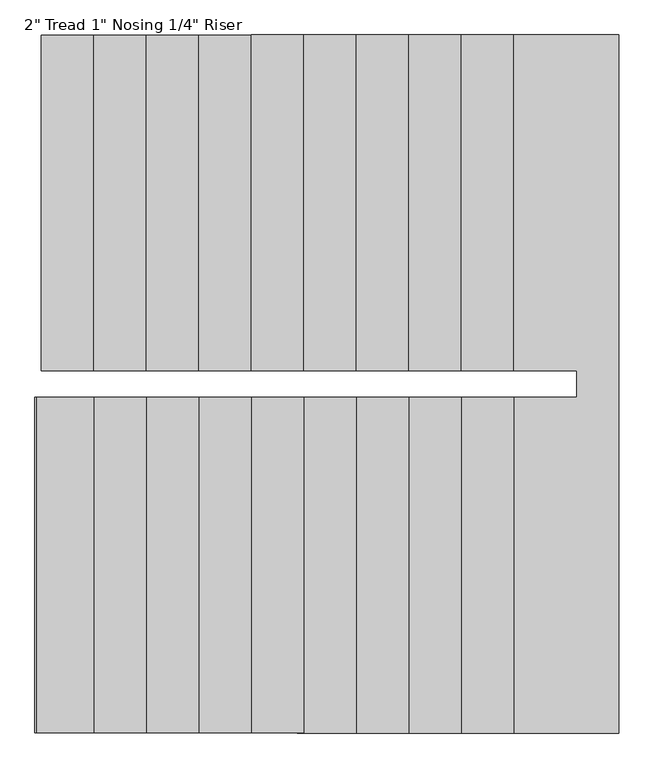
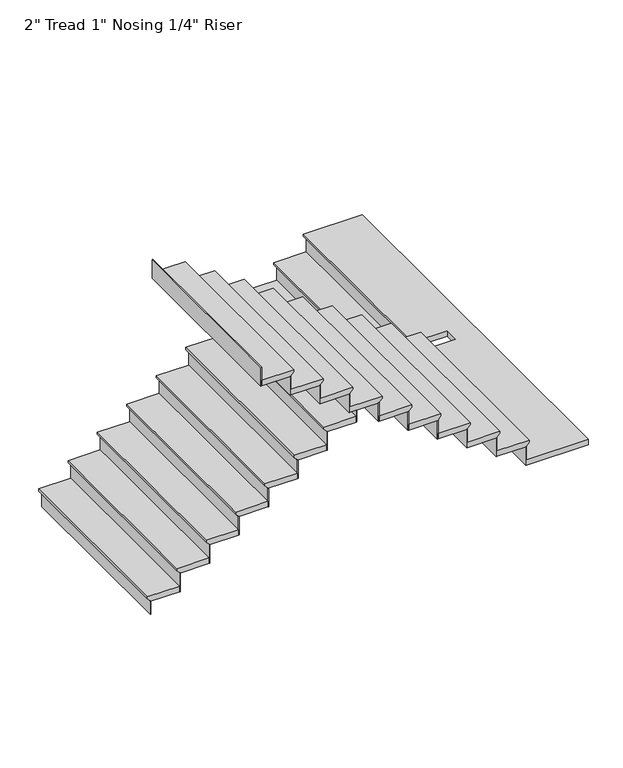
"""IFC4 building model written with IfcOpenShell, lengths in millimetres: stair flight geometry."""

from ifc_helpers import new_model, si_unit, origin, place, context, project, spatial, faceted_brep, source, transform, mapped, element, save


def stair_flight_0ebd5bc4(model_context):
    return source(origin(), model_context, "Body", "Brep", [
        faceted_brep([(-6414.1711241, 10106.9344295, 150.2833333), (-6414.1711241, 10106.9344295, 169.3333333), (-6414.1711241, 11732.5344295, 169.3333333), (-6414.1711241, 11732.5344295, 150.2833333), (-6388.7711241, 10106.9344295, 124.8833333), (-6388.7711241, 11732.5344295, 124.8833333), (-6134.7711241, 10106.9344295, 169.3333333), (-6134.7711241, 11732.5344295, 169.3333333), (-6388.7711241, 11732.5344295, 118.5333333), (-6134.7711241, 11732.5344295, 118.5333333), (-6134.7711241, 10106.9344295, 118.5333333), (-6388.7711241, 10106.9344295, 118.5333333)], [[[0, 1, 2, 3]], [[4, 0, 3, 5]], [[2, 1, 6, 7]], [[8, 9, 10, 11]], [[2, 7, 9, 8, 5, 3]], [[8, 11, 4, 5]], [[6, 1, 0, 4, 11, 10]], [[7, 6, 10, 9]]]),
        faceted_brep([(-6388.7711241, 10106.9344295, 118.5333333), (-6388.7711241, 10106.9344295, 0.0), (-6382.4211241, 10106.9344295, 0.0), (-6382.4211241, 10106.9344295, 118.5333333), (-6388.7711241, 11732.5344295, 118.5333333), (-6382.4211241, 11732.5344295, 118.5333333), (-6382.4211241, 11732.5344295, 0.0), (-6388.7711241, 11732.5344295, 0.0)], [[[0, 1, 2, 3]], [[4, 5, 6, 7]], [[1, 0, 4, 7]], [[2, 1, 7, 6]], [[3, 2, 6, 5]], [[0, 3, 5, 4]]]),
        faceted_brep([(-6134.7711241, 10106.9344295, 287.8666667), (-6134.7711241, 10106.9344295, 118.5333333), (-6128.4211241, 10106.9344295, 118.5333333), (-6128.4211241, 10106.9344295, 287.8666667), (-6134.7711241, 11732.5344295, 287.8666667), (-6128.4211241, 11732.5344295, 287.8666667), (-6128.4211241, 11732.5344295, 118.5333333), (-6134.7711241, 11732.5344295, 118.5333333)], [[[0, 1, 2, 3]], [[4, 5, 6, 7]], [[1, 0, 4, 7]], [[2, 1, 7, 6]], [[3, 2, 6, 5]], [[0, 3, 5, 4]]]),
        faceted_brep([(-6160.1711241, 11732.5344295, 338.6666667), (-6160.1711241, 10106.9344295, 338.6666667), (-5880.7711241, 10106.9344295, 338.6666667), (-5880.7711241, 11732.5344295, 338.6666667), (-6134.7711241, 11732.5344295, 287.8666667), (-5880.7711241, 11732.5344295, 287.8666667), (-5880.7711241, 10106.9344295, 287.8666667), (-6134.7711241, 10106.9344295, 287.8666667), (-6134.7711241, 11732.5344295, 294.2166667), (-6160.1711241, 11732.5344295, 319.6166667), (-6134.7711241, 10106.9344295, 294.2166667), (-6160.1711241, 10106.9344295, 319.6166667)], [[[0, 1, 2, 3]], [[4, 5, 6, 7]], [[0, 3, 5, 4, 8, 9]], [[4, 7, 10, 8]], [[2, 1, 11, 10, 7, 6]], [[3, 2, 6, 5]], [[11, 1, 0, 9]], [[10, 11, 9, 8]]]),
        faceted_brep([(-5880.7711241, 10106.9344295, 457.2), (-5880.7711241, 10106.9344295, 287.8666667), (-5874.4211241, 10106.9344295, 287.8666667), (-5874.4211241, 10106.9344295, 457.2), (-5880.7711241, 11732.5344295, 457.2), (-5874.4211241, 11732.5344295, 457.2), (-5874.4211241, 11732.5344295, 287.8666667), (-5880.7711241, 11732.5344295, 287.8666667)], [[[0, 1, 2, 3]], [[4, 5, 6, 7]], [[1, 0, 4, 7]], [[2, 1, 7, 6]], [[3, 2, 6, 5]], [[0, 3, 5, 4]]]),
        faceted_brep([(-5906.1711241, 11732.5344295, 508.0), (-5906.1711241, 10106.9344295, 508.0), (-5626.7711241, 10106.9344295, 508.0), (-5626.7711241, 11732.5344295, 508.0), (-5880.7711241, 11732.5344295, 457.2), (-5626.7711241, 11732.5344295, 457.2), (-5626.7711241, 10106.9344295, 457.2), (-5880.7711241, 10106.9344295, 457.2), (-5880.7711241, 11732.5344295, 463.55), (-5906.1711241, 11732.5344295, 488.95), (-5880.7711241, 10106.9344295, 463.55), (-5906.1711241, 10106.9344295, 488.95)], [[[0, 1, 2, 3]], [[4, 5, 6, 7]], [[0, 3, 5, 4, 8, 9]], [[4, 7, 10, 8]], [[2, 1, 11, 10, 7, 6]], [[3, 2, 6, 5]], [[11, 1, 0, 9]], [[10, 11, 9, 8]]]),
        faceted_brep([(-5626.7711241, 10106.9344295, 626.5333333), (-5626.7711241, 10106.9344295, 457.2), (-5620.4211241, 10106.9344295, 457.2), (-5620.4211241, 10106.9344295, 626.5333333), (-5626.7711241, 11732.5344295, 626.5333333), (-5620.4211241, 11732.5344295, 626.5333333), (-5620.4211241, 11732.5344295, 457.2), (-5626.7711241, 11732.5344295, 457.2)], [[[0, 1, 2, 3]], [[4, 5, 6, 7]], [[1, 0, 4, 7]], [[2, 1, 7, 6]], [[3, 2, 6, 5]], [[0, 3, 5, 4]]]),
        faceted_brep([(-5652.1711241, 11732.5344295, 677.3333333), (-5652.1711241, 10106.9344295, 677.3333333), (-5372.7711241, 10106.9344295, 677.3333333), (-5372.7711241, 11732.5344295, 677.3333333), (-5626.7711241, 11732.5344295, 626.5333333), (-5372.7711241, 11732.5344295, 626.5333333), (-5372.7711241, 10106.9344295, 626.5333333), (-5626.7711241, 10106.9344295, 626.5333333), (-5626.7711241, 11732.5344295, 632.8833333), (-5652.1711241, 11732.5344295, 658.2833333), (-5626.7711241, 10106.9344295, 632.8833333), (-5652.1711241, 10106.9344295, 658.2833333)], [[[0, 1, 2, 3]], [[4, 5, 6, 7]], [[0, 3, 5, 4, 8, 9]], [[4, 7, 10, 8]], [[2, 1, 11, 10, 7, 6]], [[3, 2, 6, 5]], [[11, 1, 0, 9]], [[10, 11, 9, 8]]]),
        faceted_brep([(-5372.7711241, 10106.9344295, 795.8666667), (-5372.7711241, 10106.9344295, 626.5333333), (-5366.4211241, 10106.9344295, 626.5333333), (-5366.4211241, 10106.9344295, 795.8666667), (-5372.7711241, 11732.5344295, 795.8666667), (-5366.4211241, 11732.5344295, 795.8666667), (-5366.4211241, 11732.5344295, 626.5333333), (-5372.7711241, 11732.5344295, 626.5333333)], [[[0, 1, 2, 3]], [[4, 5, 6, 7]], [[1, 0, 4, 7]], [[2, 1, 7, 6]], [[3, 2, 6, 5]], [[0, 3, 5, 4]]]),
        faceted_brep([(-5398.1711241, 11732.5344295, 846.6666667), (-5398.1711241, 10106.9344295, 846.6666667), (-5118.7711241, 10106.9344295, 846.6666667), (-5118.7711241, 11732.5344295, 846.6666667), (-5372.7711241, 11732.5344295, 795.8666667), (-5118.7711241, 11732.5344295, 795.8666667), (-5118.7711241, 10106.9344295, 795.8666667), (-5372.7711241, 10106.9344295, 795.8666667), (-5372.7711241, 11732.5344295, 802.2166667), (-5398.1711241, 11732.5344295, 827.6166667), (-5372.7711241, 10106.9344295, 802.2166667), (-5398.1711241, 10106.9344295, 827.6166667)], [[[0, 1, 2, 3]], [[4, 5, 6, 7]], [[0, 3, 5, 4, 8, 9]], [[4, 7, 10, 8]], [[2, 1, 11, 10, 7, 6]], [[3, 2, 6, 5]], [[11, 1, 0, 9]], [[10, 11, 9, 8]]]),
        faceted_brep([(-5118.7711241, 10106.9344295, 965.2), (-5118.7711241, 10106.9344295, 795.8666667), (-5112.4211241, 10106.9344295, 795.8666667), (-5112.4211241, 10106.9344295, 965.2), (-5118.7711241, 11732.5344295, 965.2), (-5112.4211241, 11732.5344295, 965.2), (-5112.4211241, 11732.5344295, 795.8666667), (-5118.7711241, 11732.5344295, 795.8666667)], [[[0, 1, 2, 3]], [[4, 5, 6, 7]], [[1, 0, 4, 7]], [[2, 1, 7, 6]], [[3, 2, 6, 5]], [[0, 3, 5, 4]]]),
        faceted_brep([(-5144.1711241, 11732.5344295, 1016.0), (-5144.1711241, 10106.9344295, 1016.0), (-4864.7711241, 10106.9344295, 1016.0), (-4864.7711241, 11732.5344295, 1016.0), (-5118.7711241, 11732.5344295, 965.2), (-4864.7711241, 11732.5344295, 965.2), (-4864.7711241, 10106.9344295, 965.2), (-5118.7711241, 10106.9344295, 965.2), (-5118.7711241, 11732.5344295, 971.55), (-5144.1711241, 11732.5344295, 996.95), (-5118.7711241, 10106.9344295, 971.55), (-5144.1711241, 10106.9344295, 996.95)], [[[0, 1, 2, 3]], [[4, 5, 6, 7]], [[0, 3, 5, 4, 8, 9]], [[4, 7, 10, 8]], [[2, 1, 11, 10, 7, 6]], [[3, 2, 6, 5]], [[11, 1, 0, 9]], [[10, 11, 9, 8]]]),
        faceted_brep([(-4864.7711241, 10106.9344295, 1134.5333333), (-4864.7711241, 10106.9344295, 965.2), (-4858.4211241, 10106.9344295, 965.2), (-4858.4211241, 10106.9344295, 1134.5333333), (-4864.7711241, 11732.5344295, 1134.5333333), (-4858.4211241, 11732.5344295, 1134.5333333), (-4858.4211241, 11732.5344295, 965.2), (-4864.7711241, 11732.5344295, 965.2)], [[[0, 1, 2, 3]], [[4, 5, 6, 7]], [[1, 0, 4, 7]], [[2, 1, 7, 6]], [[3, 2, 6, 5]], [[0, 3, 5, 4]]]),
        faceted_brep([(-4890.1711241, 11732.5344295, 1185.3333333), (-4890.1711241, 10106.9344295, 1185.3333333), (-4610.7711241, 10106.9344295, 1185.3333333), (-4610.7711241, 11732.5344295, 1185.3333333), (-4864.7711241, 11732.5344295, 1134.5333333), (-4610.7711241, 11732.5344295, 1134.5333333), (-4610.7711241, 10106.9344295, 1134.5333333), (-4864.7711241, 10106.9344295, 1134.5333333), (-4864.7711241, 11732.5344295, 1140.8833333), (-4890.1711241, 11732.5344295, 1166.2833333), (-4864.7711241, 10106.9344295, 1140.8833333), (-4890.1711241, 10106.9344295, 1166.2833333)], [[[0, 1, 2, 3]], [[4, 5, 6, 7]], [[0, 3, 5, 4, 8, 9]], [[4, 7, 10, 8]], [[2, 1, 11, 10, 7, 6]], [[3, 2, 6, 5]], [[11, 1, 0, 9]], [[10, 11, 9, 8]]]),
        faceted_brep([(-4610.7711241, 10106.9344295, 1303.8666667), (-4610.7711241, 10106.9344295, 1134.5333333), (-4604.4211241, 10106.9344295, 1134.5333333), (-4604.4211241, 10106.9344295, 1303.8666667), (-4610.7711241, 11732.5344295, 1303.8666667), (-4604.4211241, 11732.5344295, 1303.8666667), (-4604.4211241, 11732.5344295, 1134.5333333), (-4610.7711241, 11732.5344295, 1134.5333333)], [[[0, 1, 2, 3]], [[4, 5, 6, 7]], [[1, 0, 4, 7]], [[2, 1, 7, 6]], [[3, 2, 6, 5]], [[0, 3, 5, 4]]]),
        faceted_brep([(-4636.1711241, 11732.5344295, 1354.6666667), (-4636.1711241, 10106.9344295, 1354.6666667), (-4356.7711241, 10106.9344295, 1354.6666667), (-4356.7711241, 11732.5344295, 1354.6666667), (-4610.7711241, 11732.5344295, 1303.8666667), (-4356.7711241, 11732.5344295, 1303.8666667), (-4356.7711241, 10106.9344295, 1303.8666667), (-4610.7711241, 10106.9344295, 1303.8666667), (-4610.7711241, 11732.5344295, 1310.2166667), (-4636.1711241, 11732.5344295, 1335.6166667), (-4610.7711241, 10106.9344295, 1310.2166667), (-4636.1711241, 10106.9344295, 1335.6166667)], [[[0, 1, 2, 3]], [[4, 5, 6, 7]], [[0, 3, 5, 4, 8, 9]], [[4, 7, 10, 8]], [[2, 1, 11, 10, 7, 6]], [[3, 2, 6, 5]], [[11, 1, 0, 9]], [[10, 11, 9, 8]]]),
        faceted_brep([(-4356.7711241, 10106.9344295, 1473.2), (-4356.7711241, 10106.9344295, 1303.8666667), (-4350.4211241, 10106.9344295, 1303.8666667), (-4350.4211241, 10106.9344295, 1473.2), (-4356.7711241, 11732.5344295, 1473.2), (-4350.4211241, 11732.5344295, 1473.2), (-4350.4211241, 11732.5344295, 1303.8666667), (-4356.7711241, 11732.5344295, 1303.8666667)], [[[0, 1, 2, 3]], [[4, 5, 6, 7]], [[1, 0, 4, 7]], [[2, 1, 7, 6]], [[3, 2, 6, 5]], [[0, 3, 5, 4]]]),
        faceted_brep([(-4382.1711241, 11732.5344295, 1524.0), (-4382.1711241, 10106.9344295, 1524.0), (-4102.7711241, 10106.9344295, 1524.0), (-4102.7711241, 11732.5344295, 1524.0), (-4356.7711241, 11732.5344295, 1473.2), (-4102.7711241, 11732.5344295, 1473.2), (-4102.7711241, 10106.9344295, 1473.2), (-4356.7711241, 10106.9344295, 1473.2), (-4356.7711241, 11732.5344295, 1479.55), (-4382.1711241, 11732.5344295, 1504.95), (-4356.7711241, 10106.9344295, 1479.55), (-4382.1711241, 10106.9344295, 1504.95)], [[[0, 1, 2, 3]], [[4, 5, 6, 7]], [[0, 3, 5, 4, 8, 9]], [[4, 7, 10, 8]], [[2, 1, 11, 10, 7, 6]], [[3, 2, 6, 5]], [[11, 1, 0, 9]], [[10, 11, 9, 8]]]),
        faceted_brep([(-4102.7711241, 10106.9344295, 1642.5333333), (-4102.7711241, 10106.9344295, 1473.2), (-4096.4211241, 10106.9344295, 1473.2), (-4096.4211241, 10106.9344295, 1642.5333333), (-4102.7711241, 11732.5344295, 1642.5333333), (-4096.4211241, 11732.5344295, 1642.5333333), (-4096.4211241, 11732.5344295, 1473.2), (-4102.7711241, 11732.5344295, 1473.2)], [[[0, 1, 2, 3]], [[4, 5, 6, 7]], [[1, 0, 4, 7]], [[2, 1, 7, 6]], [[3, 2, 6, 5]], [[0, 3, 5, 4]]]),
        faceted_brep([(-4153.5711241, 8354.3344295, 1693.3333333), (-3620.1711241, 8354.3344295, 1693.3333333), (-3620.1711241, 11732.5344295, 1693.3333333), (-4128.1711241, 11732.5344295, 1693.3333333), (-4128.1711241, 10106.9344295, 1693.3333333), (-3823.3711241, 10106.9344295, 1693.3333333), (-3823.3711241, 9979.9344295, 1693.3333333), (-4153.5711241, 9979.9344295, 1693.3333333), (-3620.1711241, 8354.3344295, 1642.5333333), (-4153.5711241, 8354.3344295, 1642.5333333), (-4153.5711241, 9979.9344295, 1642.5333333), (-3823.3711241, 9979.9344295, 1642.5333333), (-3823.3711241, 10106.9344295, 1642.5333333), (-4102.7711241, 10106.9344295, 1642.5333333), (-4102.7711241, 11732.5344295, 1642.5333333), (-3620.1711241, 11732.5344295, 1642.5333333), (-4102.7711241, 11732.5344295, 1648.8833333), (-4128.1711241, 11732.5344295, 1674.2833333), (-4102.7711241, 10106.9344295, 1648.8833333), (-4128.1711241, 10106.9344295, 1674.2833333)], [[[0, 1, 2, 3, 4, 5, 6, 7]], [[8, 9, 10, 11, 12, 13, 14, 15]], [[1, 0, 9, 8]], [[2, 1, 8, 15]], [[3, 2, 15, 14, 16, 17]], [[14, 13, 18, 16]], [[5, 4, 19, 18, 13, 12]], [[6, 5, 12, 11]], [[7, 6, 11, 10]], [[0, 7, 10, 9]], [[19, 4, 3, 17]], [[18, 19, 17, 16]]]),
        faceted_brep([(-4153.5711241, 9979.9344295, 1811.8666667), (-4153.5711241, 9979.9344295, 1642.5333333), (-4159.9211241, 9979.9344295, 1642.5333333), (-4159.9211241, 9979.9344295, 1811.8666667), (-4153.5711241, 8354.3344295, 1811.8666667), (-4159.9211241, 8354.3344295, 1811.8666667), (-4159.9211241, 8354.3344295, 1642.5333333), (-4153.5711241, 8354.3344295, 1642.5333333)], [[[0, 1, 2, 3]], [[4, 5, 6, 7]], [[1, 0, 4, 7]], [[2, 1, 7, 6]], [[3, 2, 6, 5]], [[0, 3, 5, 4]]]),
        faceted_brep([(-4128.1711241, 8354.3344295, 1862.6666667), (-4128.1711241, 9979.9344295, 1862.6666667), (-4407.5711241, 9979.9344295, 1862.6666667), (-4407.5711241, 8354.3344295, 1862.6666667), (-4153.5711241, 8354.3344295, 1811.8666667), (-4407.5711241, 8354.3344295, 1811.8666667), (-4407.5711241, 9979.9344295, 1811.8666667), (-4153.5711241, 9979.9344295, 1811.8666667), (-4153.5711241, 8354.3344295, 1818.2166667), (-4128.1711241, 8354.3344295, 1843.6166667), (-4153.5711241, 9979.9344295, 1818.2166667), (-4128.1711241, 9979.9344295, 1843.6166667)], [[[0, 1, 2, 3]], [[4, 5, 6, 7]], [[0, 3, 5, 4, 8, 9]], [[4, 7, 10, 8]], [[2, 1, 11, 10, 7, 6]], [[3, 2, 6, 5]], [[11, 1, 0, 9]], [[10, 11, 9, 8]]]),
        faceted_brep([(-4407.5711241, 9979.9344295, 1981.2), (-4407.5711241, 9979.9344295, 1811.8666667), (-4413.9211241, 9979.9344295, 1811.8666667), (-4413.9211241, 9979.9344295, 1981.2), (-4407.5711241, 8354.3344295, 1981.2), (-4413.9211241, 8354.3344295, 1981.2), (-4413.9211241, 8354.3344295, 1811.8666667), (-4407.5711241, 8354.3344295, 1811.8666667)], [[[0, 1, 2, 3]], [[4, 5, 6, 7]], [[1, 0, 4, 7]], [[2, 1, 7, 6]], [[3, 2, 6, 5]], [[0, 3, 5, 4]]]),
        faceted_brep([(-4382.1711241, 8354.3344295, 2032.0), (-4382.1711241, 9979.9344295, 2032.0), (-4661.5711241, 9979.9344295, 2032.0), (-4661.5711241, 8354.3344295, 2032.0), (-4407.5711241, 8354.3344295, 1981.2), (-4661.5711241, 8354.3344295, 1981.2), (-4661.5711241, 9979.9344295, 1981.2), (-4407.5711241, 9979.9344295, 1981.2), (-4407.5711241, 8354.3344295, 1987.55), (-4382.1711241, 8354.3344295, 2012.95), (-4407.5711241, 9979.9344295, 1987.55), (-4382.1711241, 9979.9344295, 2012.95)], [[[0, 1, 2, 3]], [[4, 5, 6, 7]], [[0, 3, 5, 4, 8, 9]], [[4, 7, 10, 8]], [[2, 1, 11, 10, 7, 6]], [[3, 2, 6, 5]], [[11, 1, 0, 9]], [[10, 11, 9, 8]]]),
        faceted_brep([(-4661.5711241, 9979.9344295, 2150.5333333), (-4661.5711241, 9979.9344295, 1981.2), (-4667.9211241, 9979.9344295, 1981.2), (-4667.9211241, 9979.9344295, 2150.5333333), (-4661.5711241, 8354.3344295, 2150.5333333), (-4667.9211241, 8354.3344295, 2150.5333333), (-4667.9211241, 8354.3344295, 1981.2), (-4661.5711241, 8354.3344295, 1981.2)], [[[0, 1, 2, 3]], [[4, 5, 6, 7]], [[1, 0, 4, 7]], [[2, 1, 7, 6]], [[3, 2, 6, 5]], [[0, 3, 5, 4]]]),
        faceted_brep([(-4636.1711241, 8354.3344295, 2201.3333333), (-4636.1711241, 9979.9344295, 2201.3333333), (-4915.5711241, 9979.9344295, 2201.3333333), (-4915.5711241, 8354.3344295, 2201.3333333), (-4661.5711241, 8354.3344295, 2150.5333333), (-4915.5711241, 8354.3344295, 2150.5333333), (-4915.5711241, 9979.9344295, 2150.5333333), (-4661.5711241, 9979.9344295, 2150.5333333), (-4661.5711241, 8354.3344295, 2156.8833333), (-4636.1711241, 8354.3344295, 2182.2833333), (-4661.5711241, 9979.9344295, 2156.8833333), (-4636.1711241, 9979.9344295, 2182.2833333)], [[[0, 1, 2, 3]], [[4, 5, 6, 7]], [[0, 3, 5, 4, 8, 9]], [[4, 7, 10, 8]], [[2, 1, 11, 10, 7, 6]], [[3, 2, 6, 5]], [[11, 1, 0, 9]], [[10, 11, 9, 8]]]),
        faceted_brep([(-4915.5711241, 9979.9344295, 2319.8666667), (-4915.5711241, 9979.9344295, 2150.5333333), (-4921.9211241, 9979.9344295, 2150.5333333), (-4921.9211241, 9979.9344295, 2319.8666667), (-4915.5711241, 8354.3344295, 2319.8666667), (-4921.9211241, 8354.3344295, 2319.8666667), (-4921.9211241, 8354.3344295, 2150.5333333), (-4915.5711241, 8354.3344295, 2150.5333333)], [[[0, 1, 2, 3]], [[4, 5, 6, 7]], [[1, 0, 4, 7]], [[2, 1, 7, 6]], [[3, 2, 6, 5]], [[0, 3, 5, 4]]]),
        faceted_brep([(-4890.1711241, 8354.3344295, 2370.6666667), (-4890.1711241, 9979.9344295, 2370.6666667), (-5169.5711241, 9979.9344295, 2370.6666667), (-5169.5711241, 8354.3344295, 2370.6666667), (-4915.5711241, 8354.3344295, 2319.8666667), (-5169.5711241, 8354.3344295, 2319.8666667), (-5169.5711241, 9979.9344295, 2319.8666667), (-4915.5711241, 9979.9344295, 2319.8666667), (-4915.5711241, 8354.3344295, 2326.2166667), (-4890.1711241, 8354.3344295, 2351.6166667), (-4915.5711241, 9979.9344295, 2326.2166667), (-4890.1711241, 9979.9344295, 2351.6166667)], [[[0, 1, 2, 3]], [[4, 5, 6, 7]], [[0, 3, 5, 4, 8, 9]], [[4, 7, 10, 8]], [[2, 1, 11, 10, 7, 6]], [[3, 2, 6, 5]], [[11, 1, 0, 9]], [[10, 11, 9, 8]]]),
        faceted_brep([(-5169.5711241, 9979.9344295, 2489.2), (-5169.5711241, 9979.9344295, 2319.8666667), (-5175.9211241, 9979.9344295, 2319.8666667), (-5175.9211241, 9979.9344295, 2489.2), (-5169.5711241, 8354.3344295, 2489.2), (-5175.9211241, 8354.3344295, 2489.2), (-5175.9211241, 8354.3344295, 2319.8666667), (-5169.5711241, 8354.3344295, 2319.8666667)], [[[0, 1, 2, 3]], [[4, 5, 6, 7]], [[1, 0, 4, 7]], [[2, 1, 7, 6]], [[3, 2, 6, 5]], [[0, 3, 5, 4]]]),
        faceted_brep([(-5144.1711241, 8354.3344295, 2540.0), (-5144.1711241, 9979.9344295, 2540.0), (-5423.5711241, 9979.9344295, 2540.0), (-5423.5711241, 8354.3344295, 2540.0), (-5169.5711241, 8354.3344295, 2489.2), (-5423.5711241, 8354.3344295, 2489.2), (-5423.5711241, 9979.9344295, 2489.2), (-5169.5711241, 9979.9344295, 2489.2), (-5169.5711241, 8354.3344295, 2495.55), (-5144.1711241, 8354.3344295, 2520.95), (-5169.5711241, 9979.9344295, 2495.55), (-5144.1711241, 9979.9344295, 2520.95)], [[[0, 1, 2, 3]], [[4, 5, 6, 7]], [[0, 3, 5, 4, 8, 9]], [[4, 7, 10, 8]], [[2, 1, 11, 10, 7, 6]], [[3, 2, 6, 5]], [[11, 1, 0, 9]], [[10, 11, 9, 8]]]),
        faceted_brep([(-5423.5711241, 9979.9344295, 2658.5333333), (-5423.5711241, 9979.9344295, 2489.2), (-5429.9211241, 9979.9344295, 2489.2), (-5429.9211241, 9979.9344295, 2658.5333333), (-5423.5711241, 8354.3344295, 2658.5333333), (-5429.9211241, 8354.3344295, 2658.5333333), (-5429.9211241, 8354.3344295, 2489.2), (-5423.5711241, 8354.3344295, 2489.2)], [[[0, 1, 2, 3]], [[4, 5, 6, 7]], [[1, 0, 4, 7]], [[2, 1, 7, 6]], [[3, 2, 6, 5]], [[0, 3, 5, 4]]]),
        faceted_brep([(-5398.1711241, 8354.3344295, 2709.3333333), (-5398.1711241, 9979.9344295, 2709.3333333), (-5677.5711241, 9979.9344295, 2709.3333333), (-5677.5711241, 8354.3344295, 2709.3333333), (-5423.5711241, 8354.3344295, 2658.5333333), (-5677.5711241, 8354.3344295, 2658.5333333), (-5677.5711241, 9979.9344295, 2658.5333333), (-5423.5711241, 9979.9344295, 2658.5333333), (-5423.5711241, 8354.3344295, 2664.8833333), (-5398.1711241, 8354.3344295, 2690.2833333), (-5423.5711241, 9979.9344295, 2664.8833333), (-5398.1711241, 9979.9344295, 2690.2833333)], [[[0, 1, 2, 3]], [[4, 5, 6, 7]], [[0, 3, 5, 4, 8, 9]], [[4, 7, 10, 8]], [[2, 1, 11, 10, 7, 6]], [[3, 2, 6, 5]], [[11, 1, 0, 9]], [[10, 11, 9, 8]]]),
        faceted_brep([(-5677.5711241, 9979.9344295, 2827.8666667), (-5677.5711241, 9979.9344295, 2658.5333333), (-5683.9211241, 9979.9344295, 2658.5333333), (-5683.9211241, 9979.9344295, 2827.8666667), (-5677.5711241, 8354.3344295, 2827.8666667), (-5683.9211241, 8354.3344295, 2827.8666667), (-5683.9211241, 8354.3344295, 2658.5333333), (-5677.5711241, 8354.3344295, 2658.5333333)], [[[0, 1, 2, 3]], [[4, 5, 6, 7]], [[1, 0, 4, 7]], [[2, 1, 7, 6]], [[3, 2, 6, 5]], [[0, 3, 5, 4]]]),
        faceted_brep([(-5652.1711241, 8354.3344295, 2878.6666667), (-5652.1711241, 9979.9344295, 2878.6666667), (-5931.5711241, 9979.9344295, 2878.6666667), (-5931.5711241, 8354.3344295, 2878.6666667), (-5677.5711241, 8354.3344295, 2827.8666667), (-5931.5711241, 8354.3344295, 2827.8666667), (-5931.5711241, 9979.9344295, 2827.8666667), (-5677.5711241, 9979.9344295, 2827.8666667), (-5677.5711241, 8354.3344295, 2834.2166667), (-5652.1711241, 8354.3344295, 2859.6166667), (-5677.5711241, 9979.9344295, 2834.2166667), (-5652.1711241, 9979.9344295, 2859.6166667)], [[[0, 1, 2, 3]], [[4, 5, 6, 7]], [[0, 3, 5, 4, 8, 9]], [[4, 7, 10, 8]], [[2, 1, 11, 10, 7, 6]], [[3, 2, 6, 5]], [[11, 1, 0, 9]], [[10, 11, 9, 8]]]),
        faceted_brep([(-5931.5711241, 9979.9344295, 2997.2), (-5931.5711241, 9979.9344295, 2827.8666667), (-5937.9211241, 9979.9344295, 2827.8666667), (-5937.9211241, 9979.9344295, 2997.2), (-5931.5711241, 8354.3344295, 2997.2), (-5937.9211241, 8354.3344295, 2997.2), (-5937.9211241, 8354.3344295, 2827.8666667), (-5931.5711241, 8354.3344295, 2827.8666667)], [[[0, 1, 2, 3]], [[4, 5, 6, 7]], [[1, 0, 4, 7]], [[2, 1, 7, 6]], [[3, 2, 6, 5]], [[0, 3, 5, 4]]]),
        faceted_brep([(-5906.1711241, 8354.3344295, 3048.0), (-5906.1711241, 9979.9344295, 3048.0), (-6185.5711241, 9979.9344295, 3048.0), (-6185.5711241, 8354.3344295, 3048.0), (-5931.5711241, 8354.3344295, 2997.2), (-6185.5711241, 8354.3344295, 2997.2), (-6185.5711241, 9979.9344295, 2997.2), (-5931.5711241, 9979.9344295, 2997.2), (-5931.5711241, 8354.3344295, 3003.55), (-5906.1711241, 8354.3344295, 3028.95), (-5931.5711241, 9979.9344295, 3003.55), (-5906.1711241, 9979.9344295, 3028.95)], [[[0, 1, 2, 3]], [[4, 5, 6, 7]], [[0, 3, 5, 4, 8, 9]], [[4, 7, 10, 8]], [[2, 1, 11, 10, 7, 6]], [[3, 2, 6, 5]], [[11, 1, 0, 9]], [[10, 11, 9, 8]]]),
        faceted_brep([(-6185.5711241, 9979.9344295, 3166.5333333), (-6185.5711241, 9979.9344295, 2997.2), (-6191.9211241, 9979.9344295, 2997.2), (-6191.9211241, 9979.9344295, 3166.5333333), (-6185.5711241, 8354.3344295, 3166.5333333), (-6191.9211241, 8354.3344295, 3166.5333333), (-6191.9211241, 8354.3344295, 2997.2), (-6185.5711241, 8354.3344295, 2997.2)], [[[0, 1, 2, 3]], [[4, 5, 6, 7]], [[1, 0, 4, 7]], [[2, 1, 7, 6]], [[3, 2, 6, 5]], [[0, 3, 5, 4]]]),
        faceted_brep([(-6439.5711241, 9979.9344295, 3335.8666667), (-6439.5711241, 9979.9344295, 3166.5333333), (-6445.9211241, 9979.9344295, 3166.5333333), (-6445.9211241, 9979.9344295, 3335.8666667), (-6439.5711241, 8354.3344295, 3335.8666667), (-6445.9211241, 8354.3344295, 3335.8666667), (-6445.9211241, 8354.3344295, 3166.5333333), (-6439.5711241, 8354.3344295, 3166.5333333)], [[[0, 1, 2, 3]], [[4, 5, 6, 7]], [[1, 0, 4, 7]], [[2, 1, 7, 6]], [[3, 2, 6, 5]], [[0, 3, 5, 4]]]),
        faceted_brep([(-6160.1711241, 8354.3344295, 3217.3333333), (-6160.1711241, 9979.9344295, 3217.3333333), (-6439.5711241, 9979.9344295, 3217.3333333), (-6439.5711241, 8354.3344295, 3217.3333333), (-6185.5711241, 8354.3344295, 3166.5333333), (-6439.5711241, 8354.3344295, 3166.5333333), (-6439.5711241, 9979.9344295, 3166.5333333), (-6185.5711241, 9979.9344295, 3166.5333333), (-6185.5711241, 8354.3344295, 3172.8833333), (-6160.1711241, 8354.3344295, 3198.2833333), (-6185.5711241, 9979.9344295, 3172.8833333), (-6160.1711241, 9979.9344295, 3198.2833333)], [[[0, 1, 2, 3]], [[4, 5, 6, 7]], [[0, 3, 5, 4, 8, 9]], [[4, 7, 10, 8]], [[2, 1, 11, 10, 7, 6]], [[3, 2, 6, 5]], [[11, 1, 0, 9]], [[10, 11, 9, 8]]]),
    ])


if __name__ == "__main__":
    model = new_model("IFC4")
    model_context = context("Model", 3, world=origin())
    ifc_project = project(units=[si_unit("LENGTHUNIT", "METRE", prefix="MILLI")], contexts=[model_context])
    site = spatial("IfcSite", under=ifc_project)
    building = spatial("IfcBuilding", under=site)
    placement = place(None, origin())
    stair_flight_shape = stair_flight_0ebd5bc4(model_context)
    element("IfcStairFlight", 1, ObjectType="2\" Tread 1\" Nosing 1/4\" Riser", at=placement, inside=building, context=model_context, shape_type="MappedRepresentation", body=[
        mapped(stair_flight_shape, transform((0.0, 0.0, 0.0), x_axis=(1.0, 0.0, 0.0), y_axis=(0.0, 1.0, 0.0), z_axis=(0.0, 0.0, 1.0))),
    ])
    save(model, "model.ifc")
